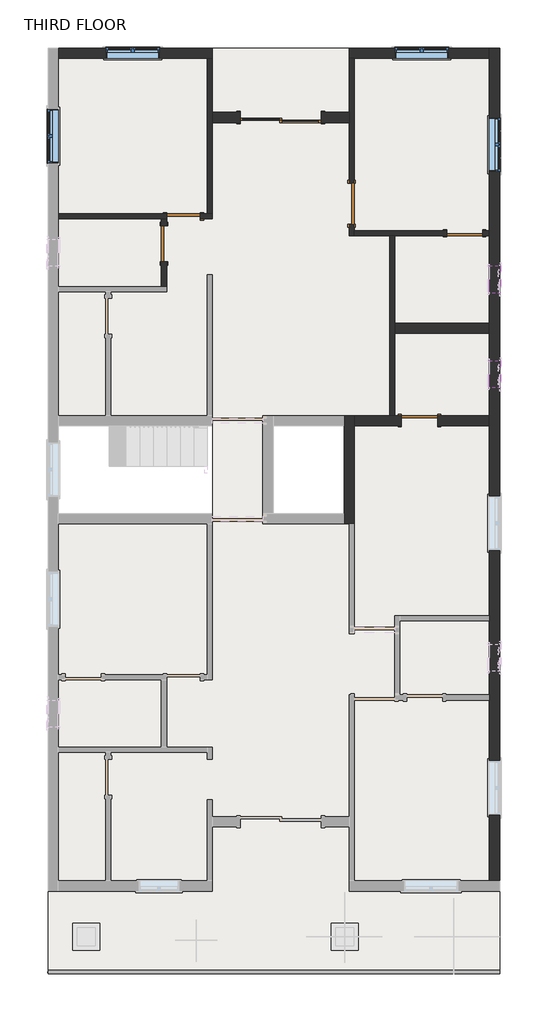
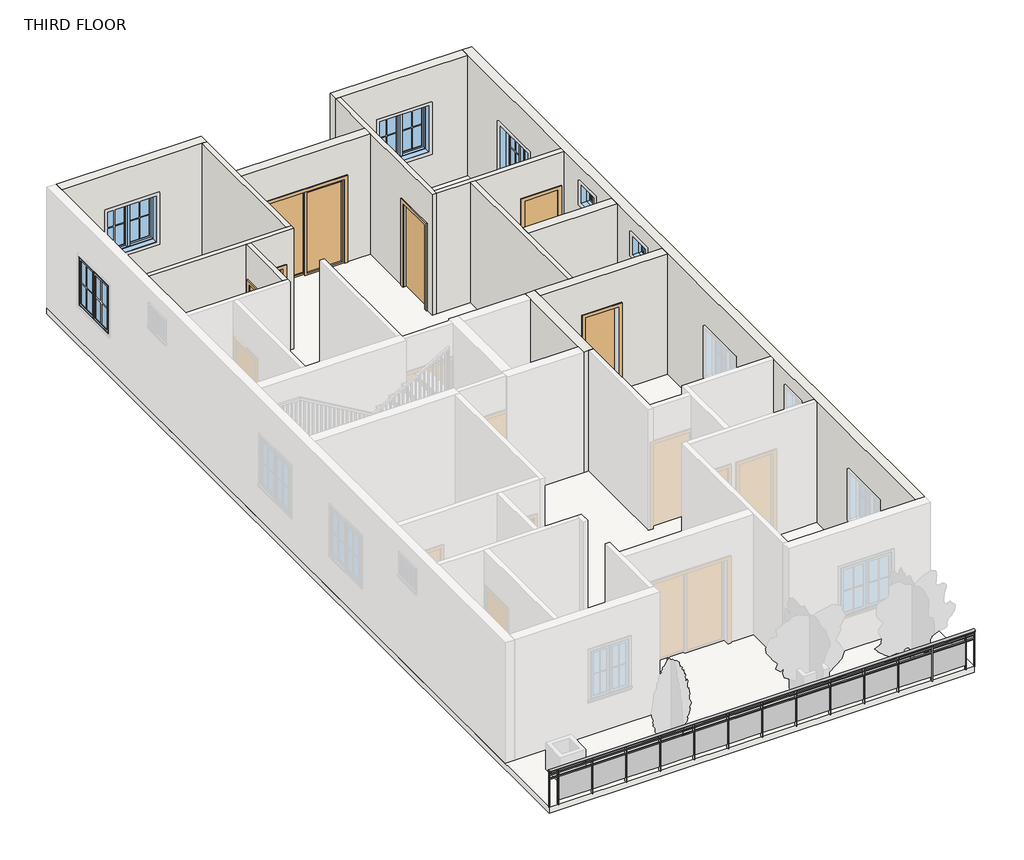
# One storey, part 2 of 4: 13 walls, 6 doors, 6 windows, 1 railing, 1 slab.
"""IFC4 building model written with IfcOpenShell, lengths in millimetres."""

from ifc_helpers import new_model, si_unit, point, frame, origin, place, context, project, spatial, polyline, ellipse_curve, trimmed, outline, extrude, faceted_brep, transform, mapped, element, save
from ifc_brep_helpers import plane_surface, extruded_surface, advanced_brep
from components import door_d4d75d1e, door_214872d5, door_d141acb4, door_38851409, door_7b345704, single_flush_3_x7_e5f9f3c4, window_79894727, window_casement_double_4_x4_af3140d2

model = new_model("IFC4")

# Units and contexts
model_context = context("Model", 3, world=origin())
ifc_project = project(units=[si_unit("LENGTHUNIT", "METRE", prefix="MILLI")], contexts=[model_context])

# Site, building, storey
site = spatial("IfcSite", under=ifc_project)
building = spatial("IfcBuilding", under=site)
storey = spatial("IfcBuildingStorey", under=building, Name="THIRD FLOOR", Elevation=9601.2)

# Doors
placement = place(None, origin())
door_shape = door_d4d75d1e(model_context)
element("IfcDoor", 1, ObjectType="Door-Double-Sliding : 72\" x 84\"", at=placement, inside=storey, context=model_context, shape_type="MappedRepresentation", body=[
    mapped(door_shape, transform((-1119.4789041, 8623.7153263, 9601.2), x_axis=(-1.0, 0.0, 0.0), y_axis=(0.0, -1.0, 0.0), z_axis=(0.0, 0.0, 1.0))),
])
door_2_shape = door_214872d5(model_context)
element("IfcDoor", 2, ObjectType="Single-Flush : 2'6\"X7'", at=placement, inside=storey, context=model_context, shape_type="MappedRepresentation", body=[
    mapped(door_2_shape, transform((-3310.2289041, 6267.8653263, 9601.2), x_axis=(1.0, 0.0, 0.0), y_axis=(0.0, 1.0, 0.0), z_axis=(0.0, 0.0, 1.0))),
])
door_3_shape = door_d141acb4(model_context)
element("IfcDoor", 3, ObjectType="Single-Flush : 2'8\"X7'", at=placement, inside=storey, context=model_context, shape_type="MappedRepresentation", body=[
    mapped(door_3_shape, transform((-3748.3789041, 5651.9153263, 9601.2), x_axis=(0.0, 1.0, 0.0), y_axis=(-1.0, 0.0, 0.0), z_axis=(0.0, 0.0, 1.0))),
])
door_4_shape = door_38851409(model_context)
element("IfcDoor", 4, ObjectType="Single-Flush : 2'8\"X7'", at=placement, inside=storey, context=model_context, shape_type="MappedRepresentation", body=[
    mapped(door_4_shape, transform((3027.0710959, 5886.8653263, 9601.2), x_axis=(1.0, 0.0, 0.0), y_axis=(0.0, 1.0, 0.0), z_axis=(0.0, 0.0, 1.0))),
])
door_5_shape = door_7b345704(model_context)
element("IfcDoor", 5, ObjectType="Single-Flush : 2'8\"X7'", at=placement, inside=storey, context=model_context, shape_type="MappedRepresentation", body=[
    mapped(door_5_shape, transform((2011.0710959, 1664.1153263, 9601.2), x_axis=(-1.0, 0.0, 0.0), y_axis=(0.0, -1.0, 0.0), z_axis=(0.0, 0.0, 1.0))),
])
single_flush_3_x7_shape = single_flush_3_x7_e5f9f3c4(model_context)
element("IfcDoor", 6, ObjectType="Single-Flush : 3'X7'", at=placement, inside=storey, context=model_context, shape_type="MappedRepresentation", body=[
    mapped(single_flush_3_x7_shape, transform((480.7210959, 6553.6153263, 9601.2), x_axis=(0.0, -1.0, 0.0), y_axis=(1.0, 0.0, 0.0), z_axis=(0.0, 0.0, 1.0))),
])

# Railing
element("IfcRailing", 7, ObjectType="Glass Panel - Bottom Fill", at=placement, inside=storey, context=model_context, shape_type="SolidModel", body=[
    advanced_brep(
    [(-6358.2289041, -10731.0846737, 10515.6), (-6358.2289041, -10807.2846737, 10515.6), (3814.4710959, -10731.0846737, 10515.6), (3814.4710959, -10807.2846737, 10515.6)],
    [
        (0, 1, ellipse_curve(frame((-6358.2289041, -10769.1846737, 10515.6), z_axis=(-1.0, 0.0, 0.0), x_axis=(0.0, -1.0, 0.0)), 38.1, 28.575)),
        (1, 0, ellipse_curve(frame((-6358.2289041, -10769.1846737, 10515.6), z_axis=(-1.0, 0.0, 0.0), x_axis=(0.0, -1.0, 0.0)), 38.1, 28.575)),
        (2, 3, ellipse_curve(frame((3814.4710959, -10769.1846737, 10515.6), z_axis=(1.0, 0.0, 0.0), x_axis=(0.0, -1.0, 0.0)), 38.1, 28.575)),
        (3, 2, ellipse_curve(frame((3814.4710959, -10769.1846737, 10515.6), z_axis=(1.0, 0.0, 0.0), x_axis=(0.0, -1.0, 0.0)), 38.1, 28.575)),
        (0, 2),
        (3, 1),
    ],
    [
        plane_surface(frame((-6358.2289041, -10769.1846737, 10515.6), z_axis=(-1.0, 0.0, 0.0), x_axis=(0.0, 1.0, 0.0))),
        plane_surface(frame((3814.4710959, -10769.1846737, 10515.6), z_axis=(1.0, 0.0, 0.0), x_axis=(0.0, 1.0, 0.0))),
        extruded_surface(trimmed(ellipse_curve(frame((3814.4710959, -10769.1846737, 10515.6), z_axis=(-1.0, 0.0, 0.0), x_axis=(0.0, -1.0, 0.0)), 38.1, 28.575), [point((3814.4710959, -10731.0846737, 10515.6))], [point((3814.4710959, -10807.2846737, 10515.6))], True, "CARTESIAN"), (-10172.7, 0.0, 0.0), 10172.7),
        extruded_surface(trimmed(ellipse_curve(frame((3814.4710959, -10769.1846737, 10515.6), z_axis=(-1.0, 0.0, 0.0), x_axis=(0.0, -1.0, 0.0)), 38.1, 28.575), [point((3814.4710959, -10807.2846737, 10515.6))], [point((3814.4710959, -10731.0846737, 10515.6))], True, "CARTESIAN"), (-10172.7, 0.0, 0.0), 10172.7),
    ],
    [
        (0, [[1, 2]]),
        (1, [[3, 4]]),
        (2, [[-1, 5, -4, 6]]),
        (3, [[-2, -6, -3, -5]]),
    ],
),
    extrude(outline(polyline([(-6358.2289041, -10781.8846737), (-6358.2289041, -10756.4846737), (3814.4710959, -10756.4846737), (3814.4710959, -10781.8846737), (-6358.2289041, -10781.8846737)])), frame((0.0, 0.0, 10401.3), z_axis=(0.0, 0.0, 1.0), x_axis=(1.0, 0.0, 0.0)), (0.0, 0.0, 1.0), 25.4),
    extrude(outline(polyline([(-6358.2289041, -10781.8846737), (-6358.2289041, -10756.4846737), (3814.4710959, -10756.4846737), (3814.4710959, -10781.8846737), (-6358.2289041, -10781.8846737)])), frame((0.0, 0.0, 10299.7), z_axis=(0.0, 0.0, 1.0), x_axis=(1.0, 0.0, 0.0)), (0.0, 0.0, 1.0), 25.4),
    extrude(outline(polyline([(3598.5710959, -10794.5846737), (3598.5710959, -10743.7846737), (3611.2710959, -10743.7846737), (3611.2710959, -10794.5846737), (3598.5710959, -10794.5846737)])), frame((0.0, 0.0, 9601.2), z_axis=(0.0, 0.0, 1.0), x_axis=(1.0, 0.0, 0.0)), (0.0, 0.0, 1.0), 885.825),
    extrude(outline(polyline([(2792.1210959, -10762.6495167), (3604.9210959, -10762.6495167), (3604.9210959, -10768.9995167), (2792.1210959, -10768.9995167), (2792.1210959, -10762.6495167)])), frame((0.0, 0.0, 9702.8), z_axis=(0.0, 0.0, 1.0), x_axis=(1.0, 0.0, 0.0)), (0.0, 0.0, 1.0), 596.9),
    extrude(outline(polyline([(2785.7710959, -10794.5846737), (2785.7710959, -10743.7846737), (2798.4710959, -10743.7846737), (2798.4710959, -10794.5846737), (2785.7710959, -10794.5846737)])), frame((0.0, 0.0, 9601.2), z_axis=(0.0, 0.0, 1.0), x_axis=(1.0, 0.0, 0.0)), (0.0, 0.0, 1.0), 885.825),
    extrude(outline(polyline([(1979.3210959, -10762.6495167), (2792.1210959, -10762.6495167), (2792.1210959, -10768.9995167), (1979.3210959, -10768.9995167), (1979.3210959, -10762.6495167)])), frame((0.0, 0.0, 9702.8), z_axis=(0.0, 0.0, 1.0), x_axis=(1.0, 0.0, 0.0)), (0.0, 0.0, 1.0), 596.9),
    extrude(outline(polyline([(1972.9710959, -10794.5846737), (1972.9710959, -10743.7846737), (1985.6710959, -10743.7846737), (1985.6710959, -10794.5846737), (1972.9710959, -10794.5846737)])), frame((0.0, 0.0, 9601.2), z_axis=(0.0, 0.0, 1.0), x_axis=(1.0, 0.0, 0.0)), (0.0, 0.0, 1.0), 885.825),
    extrude(outline(polyline([(1166.5210959, -10762.6495167), (1979.3210959, -10762.6495167), (1979.3210959, -10768.9995167), (1166.5210959, -10768.9995167), (1166.5210959, -10762.6495167)])), frame((0.0, 0.0, 9702.8), z_axis=(0.0, 0.0, 1.0), x_axis=(1.0, 0.0, 0.0)), (0.0, 0.0, 1.0), 596.9),
    extrude(outline(polyline([(1160.1710959, -10794.5846737), (1160.1710959, -10743.7846737), (1172.8710959, -10743.7846737), (1172.8710959, -10794.5846737), (1160.1710959, -10794.5846737)])), frame((0.0, 0.0, 9601.2), z_axis=(0.0, 0.0, 1.0), x_axis=(1.0, 0.0, 0.0)), (0.0, 0.0, 1.0), 885.825),
    extrude(outline(polyline([(353.7210959, -10762.6495167), (1166.5210959, -10762.6495167), (1166.5210959, -10768.9995167), (353.7210959, -10768.9995167), (353.7210959, -10762.6495167)])), frame((0.0, 0.0, 9702.8), z_axis=(0.0, 0.0, 1.0), x_axis=(1.0, 0.0, 0.0)), (0.0, 0.0, 1.0), 596.9),
    extrude(outline(polyline([(347.3710959, -10794.5846737), (347.3710959, -10743.7846737), (360.0710959, -10743.7846737), (360.0710959, -10794.5846737), (347.3710959, -10794.5846737)])), frame((0.0, 0.0, 9601.2), z_axis=(0.0, 0.0, 1.0), x_axis=(1.0, 0.0, 0.0)), (0.0, 0.0, 1.0), 885.825),
    extrude(outline(polyline([(-459.0789041, -10762.6495167), (353.7210959, -10762.6495167), (353.7210959, -10768.9995167), (-459.0789041, -10768.9995167), (-459.0789041, -10762.6495167)])), frame((0.0, 0.0, 9702.8), z_axis=(0.0, 0.0, 1.0), x_axis=(1.0, 0.0, 0.0)), (0.0, 0.0, 1.0), 596.9),
    extrude(outline(polyline([(-465.4289041, -10794.5846737), (-465.4289041, -10743.7846737), (-452.7289041, -10743.7846737), (-452.7289041, -10794.5846737), (-465.4289041, -10794.5846737)])), frame((0.0, 0.0, 9601.2), z_axis=(0.0, 0.0, 1.0), x_axis=(1.0, 0.0, 0.0)), (0.0, 0.0, 1.0), 885.825),
    extrude(outline(polyline([(-1271.8789041, -10762.6495167), (-459.0789041, -10762.6495167), (-459.0789041, -10768.9995167), (-1271.8789041, -10768.9995167), (-1271.8789041, -10762.6495167)])), frame((0.0, 0.0, 9702.8), z_axis=(0.0, 0.0, 1.0), x_axis=(1.0, 0.0, 0.0)), (0.0, 0.0, 1.0), 596.9),
    extrude(outline(polyline([(-1278.2289041, -10794.5846737), (-1278.2289041, -10743.7846737), (-1265.5289041, -10743.7846737), (-1265.5289041, -10794.5846737), (-1278.2289041, -10794.5846737)])), frame((0.0, 0.0, 9601.2), z_axis=(0.0, 0.0, 1.0), x_axis=(1.0, 0.0, 0.0)), (0.0, 0.0, 1.0), 885.825),
    extrude(outline(polyline([(-2084.6789041, -10762.6495167), (-1271.8789041, -10762.6495167), (-1271.8789041, -10768.9995167), (-2084.6789041, -10768.9995167), (-2084.6789041, -10762.6495167)])), frame((0.0, 0.0, 9702.8), z_axis=(0.0, 0.0, 1.0), x_axis=(1.0, 0.0, 0.0)), (0.0, 0.0, 1.0), 596.9),
    extrude(outline(polyline([(-2091.0289041, -10794.5846737), (-2091.0289041, -10743.7846737), (-2078.3289041, -10743.7846737), (-2078.3289041, -10794.5846737), (-2091.0289041, -10794.5846737)])), frame((0.0, 0.0, 9601.2), z_axis=(0.0, 0.0, 1.0), x_axis=(1.0, 0.0, 0.0)), (0.0, 0.0, 1.0), 885.825),
    extrude(outline(polyline([(-2897.4789041, -10762.6495167), (-2084.6789041, -10762.6495167), (-2084.6789041, -10768.9995167), (-2897.4789041, -10768.9995167), (-2897.4789041, -10762.6495167)])), frame((0.0, 0.0, 9702.8), z_axis=(0.0, 0.0, 1.0), x_axis=(1.0, 0.0, 0.0)), (0.0, 0.0, 1.0), 596.9),
    extrude(outline(polyline([(-2903.8289041, -10794.5846737), (-2903.8289041, -10743.7846737), (-2891.1289041, -10743.7846737), (-2891.1289041, -10794.5846737), (-2903.8289041, -10794.5846737)])), frame((0.0, 0.0, 9601.2), z_axis=(0.0, 0.0, 1.0), x_axis=(1.0, 0.0, 0.0)), (0.0, 0.0, 1.0), 885.825),
    extrude(outline(polyline([(-3710.2789041, -10762.6495167), (-2897.4789041, -10762.6495167), (-2897.4789041, -10768.9995167), (-3710.2789041, -10768.9995167), (-3710.2789041, -10762.6495167)])), frame((0.0, 0.0, 9702.8), z_axis=(0.0, 0.0, 1.0), x_axis=(1.0, 0.0, 0.0)), (0.0, 0.0, 1.0), 596.9),
    extrude(outline(polyline([(-3716.6289041, -10794.5846737), (-3716.6289041, -10743.7846737), (-3703.9289041, -10743.7846737), (-3703.9289041, -10794.5846737), (-3716.6289041, -10794.5846737)])), frame((0.0, 0.0, 9601.2), z_axis=(0.0, 0.0, 1.0), x_axis=(1.0, 0.0, 0.0)), (0.0, 0.0, 1.0), 885.825),
    extrude(outline(polyline([(-4523.0789041, -10762.6495167), (-3710.2789041, -10762.6495167), (-3710.2789041, -10768.9995167), (-4523.0789041, -10768.9995167), (-4523.0789041, -10762.6495167)])), frame((0.0, 0.0, 9702.8), z_axis=(0.0, 0.0, 1.0), x_axis=(1.0, 0.0, 0.0)), (0.0, 0.0, 1.0), 596.9),
    extrude(outline(polyline([(-4529.4289041, -10794.5846737), (-4529.4289041, -10743.7846737), (-4516.7289041, -10743.7846737), (-4516.7289041, -10794.5846737), (-4529.4289041, -10794.5846737)])), frame((0.0, 0.0, 9601.2), z_axis=(0.0, 0.0, 1.0), x_axis=(1.0, 0.0, 0.0)), (0.0, 0.0, 1.0), 885.825),
    extrude(outline(polyline([(-5335.8789041, -10762.6495167), (-4523.0789041, -10762.6495167), (-4523.0789041, -10768.9995167), (-5335.8789041, -10768.9995167), (-5335.8789041, -10762.6495167)])), frame((0.0, 0.0, 9702.8), z_axis=(0.0, 0.0, 1.0), x_axis=(1.0, 0.0, 0.0)), (0.0, 0.0, 1.0), 596.9),
    extrude(outline(polyline([(-5342.2289041, -10794.5846737), (-5342.2289041, -10743.7846737), (-5329.5289041, -10743.7846737), (-5329.5289041, -10794.5846737), (-5342.2289041, -10794.5846737)])), frame((0.0, 0.0, 9601.2), z_axis=(0.0, 0.0, 1.0), x_axis=(1.0, 0.0, 0.0)), (0.0, 0.0, 1.0), 885.825),
    extrude(outline(polyline([(-6148.6789041, -10762.6495167), (-5335.8789041, -10762.6495167), (-5335.8789041, -10768.9995167), (-6148.6789041, -10768.9995167), (-6148.6789041, -10762.6495167)])), frame((0.0, 0.0, 9702.8), z_axis=(0.0, 0.0, 1.0), x_axis=(1.0, 0.0, 0.0)), (0.0, 0.0, 1.0), 596.9),
    extrude(outline(polyline([(-6155.0289041, -10794.5846737), (-6155.0289041, -10743.7846737), (-6142.3289041, -10743.7846737), (-6142.3289041, -10794.5846737), (-6155.0289041, -10794.5846737)])), frame((0.0, 0.0, 9601.2), z_axis=(0.0, 0.0, 1.0), x_axis=(1.0, 0.0, 0.0)), (0.0, 0.0, 1.0), 885.825),
    extrude(outline(polyline([(3801.7710959, -10778.7096737), (3801.7710959, -10759.6596737), (3820.8210959, -10759.6596737), (3820.8210959, -10778.7096737), (3801.7710959, -10778.7096737)])), frame((0.0, 0.0, 9601.2), z_axis=(0.0, 0.0, 1.0), x_axis=(1.0, 0.0, 0.0)), (0.0, 0.0, 1.0), 885.825),
    extrude(outline(polyline([(-6364.5789041, -10778.7096737), (-6364.5789041, -10759.6596737), (-6345.5289041, -10759.6596737), (-6345.5289041, -10778.7096737), (-6364.5789041, -10778.7096737)])), frame((0.0, 0.0, 9601.2), z_axis=(0.0, 0.0, 1.0), x_axis=(1.0, 0.0, 0.0)), (0.0, 0.0, 1.0), 885.825),
])

# Slab
element("IfcSlab", 8, ObjectType="6\"", at=placement, inside=storey, context=model_context, shape_type="SweptSolid", body=[
    extrude(outline(polyline([(3814.4710959, 10058.8153263), (3814.4710959, -10769.1846737), (-6358.2289041, -10769.1846737), (-6358.2289041, 10058.8153263), (3814.4710959, 10058.8153263)]), holes=[polyline([(-2662.5289041, 1549.8153263), (-6129.6289041, 1549.8153263), (-6129.6289041, -431.3846737), (-2662.5289041, -431.3846737), (-2662.5289041, 1549.8153263)]), polyline([(537.8710959, 1778.4153263), (-1519.5289041, 1778.4153263), (-1519.5289041, -659.9846737), (537.8710959, -659.9846737), (537.8710959, 1778.4153263)])]), frame((0.0, 0.0, 9448.8), z_axis=(0.0, 0.0, 1.0), x_axis=(1.0, 0.0, 0.0)), (0.0, 0.0, 1.0), 152.4),
])

# Walls
element("IfcWall", 9, ObjectType="4.5\"", at=placement, inside=storey, context=model_context, shape_type="SweptSolid", body=[
    extrude(outline(polyline([(6210.7153263, 9601.2), (6058.3153263, 9601.2), (6058.3153263, 11734.8), (5245.5153263, 11734.8), (5245.5153263, 9601.2), (4686.7153263, 9601.2), (4686.7153263, 12649.2), (6210.7153263, 12649.2), (6210.7153263, 9601.2)])), frame((-3805.5289041, 0.0, 0.0), z_axis=(1.0, 0.0, 0.0), x_axis=(0.0, 1.0, 0.0)), (0.0, 0.0, 1.0), 114.3),
])
element("IfcWall", 10, ObjectType="4.5\"", at=placement, inside=storey, context=model_context, shape_type="Brep", body=[
    faceted_brep([(-2929.2289041, 6210.7153263, 11734.8), (-2929.2289041, 6210.7153263, 9601.2), (-2662.5289041, 6210.7153263, 9601.2), (-2662.5289041, 6210.7153263, 12649.2), (-3691.2289041, 6210.7153263, 12649.2), (-3805.5289041, 6210.7153263, 12649.2), (-6129.6289041, 6210.7153263, 12649.2), (-6129.6289041, 6210.7153263, 9601.2), (-3805.5289041, 6210.7153263, 9601.2), (-3691.2289041, 6210.7153263, 9601.2), (-3691.2289041, 6210.7153263, 11734.8), (-2662.5289041, 6325.0153263, 9601.2), (-2776.8289041, 6325.0153263, 9601.2), (-2929.2289041, 6325.0153263, 9601.2), (-2929.2289041, 6325.0153263, 11734.8), (-3691.2289041, 6325.0153263, 11734.8), (-3691.2289041, 6325.0153263, 9601.2), (-6129.6289041, 6325.0153263, 9601.2), (-6129.6289041, 6325.0153263, 12649.2), (-2776.8289041, 6325.0153263, 12649.2), (-2662.5289041, 6325.0153263, 12649.2)], [[[0, 1, 2, 3, 4, 5, 6, 7, 8, 9, 10]], [[11, 12, 13, 14, 15, 16, 17, 18, 19, 20]], [[2, 1, 13, 12, 11]], [[9, 8, 7, 17, 16]], [[6, 5, 4, 3, 20, 19, 18]], [[7, 6, 18, 17]], [[3, 2, 11, 20]], [[14, 13, 1, 0]], [[15, 14, 0, 10]], [[16, 15, 10, 9]]]),
])
element("IfcWall", 11, ObjectType="4.5\"", at=placement, inside=storey, context=model_context, shape_type="Brep", body=[
    faceted_brep([(-2662.5289041, 6325.0153263, 9601.2), (-2662.5289041, 8382.4153263, 9601.2), (-2662.5289041, 8611.0153263, 9601.2), (-2662.5289041, 9830.2153263, 9601.2), (-2662.5289041, 9830.2153263, 12649.2), (-2662.5289041, 8611.0153263, 12649.2), (-2662.5289041, 8382.4153263, 12649.2), (-2662.5289041, 6325.0153263, 12649.2), (-2776.8289041, 6325.0153263, 9601.2), (-2776.8289041, 6325.0153263, 12649.2), (-2776.8289041, 9830.2153263, 12649.2), (-2776.8289041, 9830.2153263, 9601.2)], [[[0, 1, 2, 3, 4, 5, 6, 7]], [[8, 9, 10, 11]], [[3, 2, 1, 0, 8, 11]], [[7, 6, 5, 4, 10, 9]], [[0, 7, 9, 8]], [[4, 3, 11, 10]]]),
])
element("IfcWall", 12, ObjectType="4.5\"", at=placement, inside=storey, context=model_context, shape_type="Brep", body=[
    faceted_brep([(423.5710959, 6096.4153263, 11734.8), (423.5710959, 6096.4153263, 9601.2), (423.5710959, 5829.7153263, 9601.2), (423.5710959, 5829.7153263, 12649.2), (423.5710959, 8382.4153263, 12649.2), (423.5710959, 8611.0153263, 12649.2), (423.5710959, 9830.2153263, 12649.2), (423.5710959, 9830.2153263, 9601.2), (423.5710959, 8611.0153263, 9601.2), (423.5710959, 8382.4153263, 9601.2), (423.5710959, 7010.8153263, 9601.2), (423.5710959, 7010.8153263, 11734.8), (537.8710959, 5829.7153263, 9601.2), (537.8710959, 5944.0153263, 9601.2), (537.8710959, 6096.4153263, 9601.2), (537.8710959, 6096.4153263, 11734.8), (537.8710959, 7010.8153263, 11734.8), (537.8710959, 7010.8153263, 9601.2), (537.8710959, 9830.2153263, 9601.2), (537.8710959, 9830.2153263, 12649.2), (537.8710959, 5944.0153263, 12649.2), (537.8710959, 5829.7153263, 12649.2)], [[[0, 1, 2, 3, 4, 5, 6, 7, 8, 9, 10, 11]], [[12, 13, 14, 15, 16, 17, 18, 19, 20, 21]], [[2, 1, 14, 13, 12]], [[10, 9, 8, 7, 18, 17]], [[6, 5, 4, 3, 21, 20, 19]], [[7, 6, 19, 18]], [[3, 2, 12, 21]], [[15, 14, 1, 0]], [[16, 15, 0, 11]], [[17, 16, 11, 10]]]),
])
element("IfcWall", 13, ObjectType="4.5\"", at=placement, inside=storey, context=model_context, shape_type="Brep", body=[
    faceted_brep([(3433.4710959, 5829.7153263, 11734.8), (3433.4710959, 5829.7153263, 9601.2), (3585.8710959, 5829.7153263, 9601.2), (3585.8710959, 5829.7153263, 12649.2), (1452.2710959, 5829.7153263, 12649.2), (1337.9710959, 5829.7153263, 12649.2), (537.8710959, 5829.7153263, 12649.2), (537.8710959, 5829.7153263, 9601.2), (1337.9710959, 5829.7153263, 9601.2), (1452.2710959, 5829.7153263, 9601.2), (2620.6710959, 5829.7153263, 9601.2), (2620.6710959, 5829.7153263, 11734.8), (3585.8710959, 5944.0153263, 9601.2), (3433.4710959, 5944.0153263, 9601.2), (3433.4710959, 5944.0153263, 11734.8), (2620.6710959, 5944.0153263, 11734.8), (2620.6710959, 5944.0153263, 9601.2), (537.8710959, 5944.0153263, 9601.2), (537.8710959, 5944.0153263, 12649.2), (3585.8710959, 5944.0153263, 12649.2)], [[[0, 1, 2, 3, 4, 5, 6, 7, 8, 9, 10, 11]], [[12, 13, 14, 15, 16, 17, 18, 19]], [[2, 1, 13, 12]], [[10, 9, 8, 7, 17, 16]], [[6, 5, 4, 3, 19, 18]], [[7, 6, 18, 17]], [[3, 2, 12, 19]], [[14, 13, 1, 0]], [[15, 14, 0, 11]], [[16, 15, 11, 10]]]),
])
element("IfcWall", 14, ObjectType="4.5\"", at=placement, inside=storey, context=model_context, shape_type="Brep", body=[
    faceted_brep([(1337.9710959, 5829.7153263, 9601.2), (1337.9710959, 1778.4153263, 9601.2), (1337.9710959, 1778.4153263, 12649.2), (1337.9710959, 5829.7153263, 12649.2), (1452.2710959, 5829.7153263, 9601.2), (1452.2710959, 5829.7153263, 12649.2), (1452.2710959, 3861.2153263, 12649.2), (1452.2710959, 3632.6153263, 12649.2), (1452.2710959, 1778.4153263, 12649.2), (1452.2710959, 1778.4153263, 9601.2), (1452.2710959, 3632.6153263, 9601.2), (1452.2710959, 3861.2153263, 9601.2)], [[[0, 1, 2, 3]], [[4, 5, 6, 7, 8, 9, 10, 11]], [[1, 0, 4, 11, 10, 9]], [[3, 2, 8, 7, 6, 5]], [[2, 1, 9, 8]], [[0, 3, 5, 4]]]),
])
element("IfcWall", 15, ObjectType="9\"", at=placement, inside=storey, context=model_context, shape_type="Brep", body=[
    faceted_brep([(3814.4710959, -8711.7846737, 9601.2), (3814.4710959, 10058.8153263, 9601.2), (3814.4710959, 10058.8153263, 12649.2), (3814.4710959, -8711.7846737, 12649.2), (3814.4710959, -7225.8846737, 11734.8), (3814.4710959, -6006.6846737, 11734.8), (3814.4710959, -6006.6846737, 10515.6), (3814.4710959, -7225.8846737, 10515.6), (3814.4710959, -1256.8846737, 11734.8), (3814.4710959, -37.6846737, 11734.8), (3814.4710959, -37.6846737, 10515.6), (3814.4710959, -1256.8846737, 10515.6), (3814.4710959, 7277.5153263, 11734.8), (3814.4710959, 8496.7153263, 11734.8), (3814.4710959, 8496.7153263, 10515.6), (3814.4710959, 7277.5153263, 10515.6), (3814.4710959, -3987.3846737, 12268.2), (3814.4710959, -3377.7846737, 12268.2), (3814.4710959, -3377.7846737, 11734.8), (3814.4710959, -3987.3846737, 11734.8), (3814.4710959, 2400.7153263, 12268.2), (3814.4710959, 3010.3153263, 12268.2), (3814.4710959, 3010.3153263, 11734.8), (3814.4710959, 2400.7153263, 11734.8), (3814.4710959, 4540.6653263, 12268.2), (3814.4710959, 5150.2653263, 12268.2), (3814.4710959, 5150.2653263, 11734.8), (3814.4710959, 4540.6653263, 11734.8), (3585.8710959, -8711.7846737, 9601.2), (3585.8710959, -8711.7846737, 12649.2), (3585.8710959, -4635.0846737, 12649.2), (3585.8710959, -4520.7846737, 12649.2), (3585.8710959, -2844.3846737, 12649.2), (3585.8710959, -2730.0846737, 12649.2), (3585.8710959, 1549.8153263, 12649.2), (3585.8710959, 1778.4153263, 12649.2), (3585.8710959, 3632.6153263, 12649.2), (3585.8710959, 3861.2153263, 12649.2), (3585.8710959, 5829.7153263, 12649.2), (3585.8710959, 5944.0153263, 12649.2), (3585.8710959, 9830.2153263, 12649.2), (3585.8710959, 10058.8153263, 12649.2), (3585.8710959, 10058.8153263, 9601.2), (3585.8710959, 9830.2153263, 9601.2), (3585.8710959, 5944.0153263, 9601.2), (3585.8710959, 5829.7153263, 9601.2), (3585.8710959, 3861.2153263, 9601.2), (3585.8710959, 3632.6153263, 9601.2), (3585.8710959, 1778.4153263, 9601.2), (3585.8710959, 1549.8153263, 9601.2), (3585.8710959, -2730.0846737, 9601.2), (3585.8710959, -2844.3846737, 9601.2), (3585.8710959, -4520.7846737, 9601.2), (3585.8710959, -4635.0846737, 9601.2), (3585.8710959, -7225.8846737, 11734.8), (3585.8710959, -7225.8846737, 10515.6), (3585.8710959, -6006.6846737, 10515.6), (3585.8710959, -6006.6846737, 11734.8), (3585.8710959, -1256.8846737, 11734.8), (3585.8710959, -1256.8846737, 10515.6), (3585.8710959, -37.6846737, 10515.6), (3585.8710959, -37.6846737, 11734.8), (3585.8710959, 7277.5153263, 11734.8), (3585.8710959, 7277.5153263, 10515.6), (3585.8710959, 8496.7153263, 10515.6), (3585.8710959, 8496.7153263, 11734.8), (3585.8710959, -3987.3846737, 12268.2), (3585.8710959, -3987.3846737, 11734.8), (3585.8710959, -3377.7846737, 11734.8), (3585.8710959, -3377.7846737, 12268.2), (3585.8710959, 2400.7153263, 12268.2), (3585.8710959, 2400.7153263, 11734.8), (3585.8710959, 3010.3153263, 11734.8), (3585.8710959, 3010.3153263, 12268.2), (3585.8710959, 4540.6653263, 12268.2), (3585.8710959, 4540.6653263, 11734.8), (3585.8710959, 5150.2653263, 11734.8), (3585.8710959, 5150.2653263, 12268.2)], [[[0, 1, 2, 3], [4, 5, 6, 7], [8, 9, 10, 11], [12, 13, 14, 15], [16, 17, 18, 19], [20, 21, 22, 23], [24, 25, 26, 27]], [[28, 29, 30, 31, 32, 33, 34, 35, 36, 37, 38, 39, 40, 41, 42, 43, 44, 45, 46, 47, 48, 49, 50, 51, 52, 53], [54, 55, 56, 57], [58, 59, 60, 61], [62, 63, 64, 65], [66, 67, 68, 69], [70, 71, 72, 73], [74, 75, 76, 77]], [[1, 0, 28, 53, 52, 51, 50, 49, 48, 47, 46, 45, 44, 43, 42]], [[3, 2, 41, 40, 39, 38, 37, 36, 35, 34, 33, 32, 31, 30, 29]], [[0, 3, 29, 28]], [[2, 1, 42, 41]], [[55, 54, 4, 7]], [[56, 55, 7, 6]], [[57, 56, 6, 5]], [[54, 57, 5, 4]], [[59, 58, 8, 11]], [[60, 59, 11, 10]], [[61, 60, 10, 9]], [[58, 61, 9, 8]], [[63, 62, 12, 15]], [[64, 63, 15, 14]], [[65, 64, 14, 13]], [[62, 65, 13, 12]], [[67, 66, 16, 19]], [[68, 67, 19, 18]], [[69, 68, 18, 17]], [[66, 69, 17, 16]], [[71, 70, 20, 23]], [[72, 71, 23, 22]], [[73, 72, 22, 21]], [[70, 73, 21, 20]], [[75, 74, 24, 27]], [[76, 75, 27, 26]], [[77, 76, 26, 25]], [[74, 77, 25, 24]]]),
])
element("IfcWall", 16, ObjectType="9\"", at=placement, inside=storey, context=model_context, shape_type="Brep", body=[
    faceted_brep([(3585.8710959, 10058.8153263, 9601.2), (423.5710959, 10058.8153263, 9601.2), (423.5710959, 10058.8153263, 12649.2), (3585.8710959, 10058.8153263, 12649.2), (2671.4710959, 10058.8153263, 11734.8), (1452.2710959, 10058.8153263, 11734.8), (1452.2710959, 10058.8153263, 10515.6), (2671.4710959, 10058.8153263, 10515.6), (3585.8710959, 9830.2153263, 9601.2), (3585.8710959, 9830.2153263, 12649.2), (537.8710959, 9830.2153263, 12649.2), (423.5710959, 9830.2153263, 12649.2), (423.5710959, 9830.2153263, 9601.2), (537.8710959, 9830.2153263, 9601.2), (2671.4710959, 9830.2153263, 11734.8), (2671.4710959, 9830.2153263, 10515.6), (1452.2710959, 9830.2153263, 10515.6), (1452.2710959, 9830.2153263, 11734.8)], [[[0, 1, 2, 3], [4, 5, 6, 7]], [[8, 9, 10, 11, 12, 13], [14, 15, 16, 17]], [[1, 0, 8, 13, 12]], [[3, 2, 11, 10, 9]], [[0, 3, 9, 8]], [[2, 1, 12, 11]], [[15, 14, 4, 7]], [[16, 15, 7, 6]], [[17, 16, 6, 5]], [[14, 17, 5, 4]]]),
])
element("IfcWall", 17, ObjectType="9\"", at=placement, inside=storey, context=model_context, shape_type="Brep", body=[
    faceted_brep([(-2662.5289041, 10058.8153263, 9601.2), (-6129.6289041, 10058.8153263, 9601.2), (-6129.6289041, 10058.8153263, 12649.2), (-2662.5289041, 10058.8153263, 12649.2), (-3843.6289041, 10058.8153263, 11734.8), (-5062.8289041, 10058.8153263, 11734.8), (-5062.8289041, 10058.8153263, 10515.6), (-3843.6289041, 10058.8153263, 10515.6), (-2662.5289041, 9830.2153263, 9601.2), (-2662.5289041, 9830.2153263, 12649.2), (-2776.8289041, 9830.2153263, 12649.2), (-6129.6289041, 9830.2153263, 12649.2), (-6129.6289041, 9830.2153263, 9601.2), (-2776.8289041, 9830.2153263, 9601.2), (-3843.6289041, 9830.2153263, 11734.8), (-3843.6289041, 9830.2153263, 10515.6), (-5062.8289041, 9830.2153263, 10515.6), (-5062.8289041, 9830.2153263, 11734.8)], [[[0, 1, 2, 3], [4, 5, 6, 7]], [[8, 9, 10, 11, 12, 13], [14, 15, 16, 17]], [[1, 0, 8, 13, 12]], [[3, 2, 11, 10, 9]], [[2, 1, 12, 11]], [[0, 3, 9, 8]], [[15, 14, 4, 7]], [[16, 15, 7, 6]], [[17, 16, 6, 5]], [[14, 17, 5, 4]]]),
])
element("IfcWall", 18, ObjectType="9\"", at=placement, inside=storey, context=model_context, shape_type="Brep", body=[
    faceted_brep([(309.2710959, 1778.4153263, 9601.2), (309.2710959, 1549.8153263, 9601.2), (309.2710959, -431.3846737, 9601.2), (309.2710959, -659.9846737, 9601.2), (309.2710959, -659.9846737, 12649.2), (309.2710959, -431.3846737, 12649.2), (309.2710959, 1549.8153263, 12649.2), (309.2710959, 1778.4153263, 12649.2), (537.8710959, 1778.4153263, 9601.2), (537.8710959, 1778.4153263, 12649.2), (537.8710959, 1549.8153263, 12649.2), (537.8710959, -659.9846737, 12649.2), (537.8710959, -659.9846737, 9601.2), (537.8710959, 1549.8153263, 9601.2), (423.5710959, -659.9846737, 9601.2), (423.5710959, -659.9846737, 12649.2)], [[[0, 1, 2, 3, 4, 5, 6, 7]], [[8, 9, 10, 11, 12, 13]], [[3, 2, 1, 0, 8, 13, 12, 14]], [[7, 6, 5, 4, 15, 11, 10, 9]], [[4, 3, 14, 12, 11, 15]], [[0, 7, 9, 8]]]),
])
element("IfcWall", 19, ObjectType="9\"", at=placement, inside=storey, context=model_context, shape_type="Brep", body=[
    faceted_brep([(537.8710959, 1549.8153263, 9601.2), (1604.6710959, 1549.8153263, 9601.2), (1604.6710959, 1549.8153263, 11734.8), (2417.4710959, 1549.8153263, 11734.8), (2417.4710959, 1549.8153263, 9601.2), (3585.8710959, 1549.8153263, 9601.2), (3585.8710959, 1549.8153263, 12649.2), (537.8710959, 1549.8153263, 12649.2), (1604.6710959, 1778.4153263, 11734.8), (1604.6710959, 1778.4153263, 9601.2), (1452.2710959, 1778.4153263, 9601.2), (1337.9710959, 1778.4153263, 9601.2), (537.8710959, 1778.4153263, 9601.2), (537.8710959, 1778.4153263, 12649.2), (1337.9710959, 1778.4153263, 12649.2), (1452.2710959, 1778.4153263, 12649.2), (3585.8710959, 1778.4153263, 12649.2), (3585.8710959, 1778.4153263, 9601.2), (2417.4710959, 1778.4153263, 9601.2), (2417.4710959, 1778.4153263, 11734.8)], [[[0, 1, 2, 3, 4, 5, 6, 7]], [[8, 9, 10, 11, 12, 13, 14, 15, 16, 17, 18, 19]], [[18, 17, 5, 4]], [[12, 11, 10, 9, 1, 0]], [[7, 6, 16, 15, 14, 13]], [[0, 7, 13, 12]], [[6, 5, 17, 16]], [[2, 1, 9, 8]], [[3, 2, 8, 19]], [[4, 3, 19, 18]]]),
])
element("IfcWall", 20, ObjectType="9\"", at=placement, inside=storey, context=model_context, shape_type="SweptSolid", body=[
    extrude(outline(polyline([(1452.2710959, 3861.2153263), (3585.8710959, 3861.2153263), (3585.8710959, 3632.6153263), (1452.2710959, 3632.6153263), (1452.2710959, 3861.2153263)])), frame((0.0, 0.0, 9601.2), z_axis=(0.0, 0.0, 1.0), x_axis=(1.0, 0.0, 0.0)), (0.0, 0.0, 1.0), 3048.0),
])
element("IfcWall", 21, ObjectType="9\"", at=placement, inside=storey, context=model_context, shape_type="SweptSolid", body=[
    extrude(outline(polyline([(9601.2, -2662.5289041), (9601.2, -2033.8789041), (11734.8, -2033.8789041), (11734.8, -205.0789041), (9601.2, -205.0789041), (9601.2, 423.5710959), (12649.2, 423.5710959), (12649.2, -2662.5289041), (9601.2, -2662.5289041)])), frame((0.0, 8382.4153263, 0.0), z_axis=(0.0, 1.0, 0.0), x_axis=(0.0, 0.0, 1.0)), (0.0, 0.0, 1.0), 228.6),
])

# Windows
window_shape = window_79894727(model_context)
element("IfcWindow", 22, ObjectType="Window-Casement-Double : 2'X1'9\"", at=placement, inside=storey, context=model_context, shape_type="MappedRepresentation", body=[
    mapped(window_shape, transform((3700.1710959, 2705.5153263, 9601.2), x_axis=(0.0, -1.0, 0.0), y_axis=(1.0, 0.0, 0.0), z_axis=(0.0, 0.0, 1.0))),
])
element("IfcWindow", 23, ObjectType="Window-Casement-Double : 2'X1'9\"", at=placement, inside=storey, context=model_context, shape_type="MappedRepresentation", body=[
    mapped(window_shape, transform((3700.1710959, 4845.4653263, 9601.2), x_axis=(0.0, -1.0, 0.0), y_axis=(1.0, 0.0, 0.0), z_axis=(0.0, 0.0, 1.0))),
])
window_casement_double_4_x4_shape = window_casement_double_4_x4_af3140d2(model_context)
element("IfcWindow", 24, ObjectType="Window-Casement-Double : 4'X4'", at=placement, inside=storey, context=model_context, shape_type="MappedRepresentation", body=[
    mapped(window_casement_double_4_x4_shape, transform((-4453.2289041, 9944.5153263, 9601.2), x_axis=(1.0, 0.0, 0.0), y_axis=(0.0, 1.0, 0.0), z_axis=(0.0, 0.0, 1.0))),
])
element("IfcWindow", 25, ObjectType="Window-Casement-Double : 4'X4'", at=placement, inside=storey, context=model_context, shape_type="MappedRepresentation", body=[
    mapped(window_casement_double_4_x4_shape, transform((-6243.9289041, 8077.6153263, 9601.2), x_axis=(0.0, 1.0, 0.0), y_axis=(-1.0, 0.0, 0.0), z_axis=(0.0, 0.0, 1.0))),
])
element("IfcWindow", 26, ObjectType="Window-Casement-Double : 4'X4'", at=placement, inside=storey, context=model_context, shape_type="MappedRepresentation", body=[
    mapped(window_casement_double_4_x4_shape, transform((3700.1710959, 7887.1153263, 9601.2), x_axis=(0.0, -1.0, 0.0), y_axis=(1.0, 0.0, 0.0), z_axis=(0.0, 0.0, 1.0))),
])
element("IfcWindow", 27, ObjectType="Window-Casement-Double : 4'X4'", at=placement, inside=storey, context=model_context, shape_type="MappedRepresentation", body=[
    mapped(window_casement_double_4_x4_shape, transform((2061.8710959, 9944.5153263, 9601.2), x_axis=(1.0, 0.0, 0.0), y_axis=(0.0, 1.0, 0.0), z_axis=(0.0, 0.0, 1.0))),
])

save(model, "model.ifc")

# Revit data of these elements
# Type "Door-Double-Sliding : 72\" x 84\""
#   Type Mark = "14"
#   Construction Type Id = "opn-d45"
#   Assembly Code = "C1020"
#   Analytic Construction = "Wood frame, double glass door "
#   Thickness = 0' - 2"
#   Thermal Resistance (R) = 1.8150 (h·ft²·°F)/BTU
#   Heat Transfer Coefficient (U) = 0.5510 BTU/(h·ft²·°F)
#   Height = 7' - 0"
#   Rail Width = 0' - 2"
#   Stiles = 0' - 2"
#   Trim Projection Ext = 0' - 1"
#   Trim Projection Int = 0' - 1"
#   Trim Width = 0' - 3"
#   Width = 6' - 0"
#   Define Thermal Properties by = 1
#   Glazing = Glass
#   Panel Material = Wood - Birch - Solid Stained Light Low Gloss
#   Trim Material = Paint - Sienna
#   Visual Light Transmittance = 0
#   Solar Heat Gain Coefficient = 0
#   Function = (empty or 0)
#   Wall Closure = (empty or 0)
# Type "Single-Flush : 2'6\"X7'"
#   Type Mark = "13"
#   Construction Type Id = "MDOOR"
#   Assembly Code = "C1020"
#   Analytic Construction = "Metal"
#   Thickness = 0' - 2"
#   Heat Transfer Coefficient (U) = 0.651978 BTU/(h·ft²·°F)
#   Height = 7' - 0"
#   Trim Projection Ext = 0' - 1"
#   Trim Projection Int = 0' - 1"
#   Trim Width = 0' - 3"
#   Width = 2' - 6"
#   Define Thermal Properties by = 1
#   Door Material = Door - Panel
#   Frame Material = Door - Frame
#   Visual Light Transmittance = 0
#   Solar Heat Gain Coefficient = 0
#   Function = (empty or 0)
#   Wall Closure = (empty or 0)
# Type "Single-Flush : 2'8\"X7'"
#   Type Mark = "12"
#   Construction Type Id = "MDOOR"
#   Assembly Code = "C1020"
#   Analytic Construction = "Metal"
#   Thickness = 0' - 2"
#   Heat Transfer Coefficient (U) = 0.651978 BTU/(h·ft²·°F)
#   Height = 7' - 0"
#   Trim Projection Ext = 0' - 1"
#   Trim Projection Int = 0' - 1"
#   Trim Width = 0' - 3"
#   Width = 2' - 8"
#   Define Thermal Properties by = 1
#   Door Material = Door - Panel
#   Frame Material = Door - Frame
#   Visual Light Transmittance = 0
#   Solar Heat Gain Coefficient = 0
#   Function = (empty or 0)
#   Wall Closure = (empty or 0)
# Type "Single-Flush : 3'X7'"
#   Type Mark = "8"
#   Construction Type Id = "MDOOR"
#   Assembly Code = "C1020"
#   Analytic Construction = "Metal"
#   Thickness = 0' - 2"
#   Heat Transfer Coefficient (U) = 0.651978 BTU/(h·ft²·°F)
#   Height = 7' - 0"
#   Trim Projection Ext = 0' - 1"
#   Trim Projection Int = 0' - 1"
#   Trim Width = 0' - 3"
#   Width = 3' - 0"
#   Define Thermal Properties by = 1
#   Door Material = Door - Panel
#   Frame Material = Door - Frame
#   Visual Light Transmittance = 0
#   Solar Heat Gain Coefficient = 0
#   Function = (empty or 0)
#   Wall Closure = (empty or 0)
# Type "Glass Panel - Bottom Fill"
#   Assembly Code = "C2010400"
#   built-in parameter 1008612 = 0.0416667 (stored number, unit not read)
#   built-in parameter 1008611 = 0.0416667 (stored number, unit not read)
#   built-in parameter 1008609 = 0.333333 (stored number, unit not read)
#   built-in parameter 1008604 = 0.166667 (stored number, unit not read)
#   built-in parameter 1008603 = 0.166667 (stored number, unit not read)
#   Railing Height = 3' - 0"
#   built-in parameter 1008630 = 2
#   built-in parameter 1008610 = 2
#   built-in parameter 1008618 = Baluster - Square : 3/4"
# Type "6\""
#   Assembly Code = "B1010"
#   Function = 0
#   Layers, outside or top first: 0' - 6" no material (function 1)
# Type "4.5\""
#   Assembly Code = "B2010"
#   Layers, outside or top first: 0' - 4 1/2" no material (function 1)
# Type "9\""
#   Assembly Code = "B2010"
#   Layers, outside or top first: 0' - 9" "WALL" (function 1)
# Type "Window-Casement-Double : 2'X1'9\""
#   Type Mark = "22"
#   Fire Rating = "0.5h"
#   Assembly Code = "B2020100"
#   Analytic Construction = "Double glazing - domestic"
#   Frame Extension [instance default] = 0' - 0 1/4"
#   Window Inset [instance default] = 0' - 0"
#   Wall Thickness [instance default] = 0' - 6"
#   Interior Wall Closure [instance default] = 0' - 2 1/4"
#   Half Width = 1' - 0"
#   Visual Light Transmittance = 0.81
#   Thermal Resistance (R) = 1.8146 (h·ft²·°F)/BTU
#   Solar Heat Gain Coefficient = 0.76
#   Rough Width = 2' - 0 1/2"
#   Rough Height = 1' - 9 1/2"
#   Height = 1' - 9"
#   Heat Transfer Coefficient (U) = 0.5511 BTU/(h·ft²·°F)
#   Exterior Wall Closure [instance default] = 0' - 1 1/4"
#   Extension Jamb [instance default] = 0' - 2 1/4"
#   Default Sill Height = 7' - 0"
#   Width = 2' - 0"
#   Muntin Visibility = yes
#   Interior Trim Visibility [instance default] = yes
#   Exterior Trim Visibility [instance default] = yes
#   Extension Jamb Visibility [instance default] = yes
#   Interior Trim Material = Wood - Stained
#   Muntin Pattern = Muntin Pattern_2x2 : Muntin Pattern_2x2
#   Interior Trim = Trim-Window-Interior-Flat : Picture Frame
#   Interior Frame Material = Wood - Stained
#   Glass Panel Material = Glass
#   Exterior Trim Material = Clad - White
#   Exterior Trim = Trim-Window-Exterior-Flat : with Sill
#   Exterior Frame Material = Clad - White
#   Wall Closure = (empty or 0)
# Type "Window-Casement-Double : 4'X4'"
#   Type Mark = "20"
#   Fire Rating = "0.5h"
#   Assembly Code = "B2020100"
#   Analytic Construction = "Double glazing - domestic"
#   Frame Extension [instance default] = 0' - 0 1/4"
#   Window Inset [instance default] = 0' - 0"
#   Wall Thickness [instance default] = 0' - 6"
#   Interior Wall Closure [instance default] = 0' - 2 1/4"
#   Half Width = 2' - 0"
#   Visual Light Transmittance = 0.81
#   Thermal Resistance (R) = 1.8146 (h·ft²·°F)/BTU
#   Solar Heat Gain Coefficient = 0.76
#   Rough Width = 4' - 0 1/2"
#   Rough Height = 4' - 0 1/2"
#   Height = 4' - 0"
#   Heat Transfer Coefficient (U) = 0.5511 BTU/(h·ft²·°F)
#   Exterior Wall Closure [instance default] = 0' - 1 1/4"
#   Extension Jamb [instance default] = 0' - 2 1/4"
#   Default Sill Height = 3' - 0"
#   Width = 4' - 0"
#   Muntin Visibility = yes
#   Interior Trim Visibility [instance default] = yes
#   Exterior Trim Visibility [instance default] = yes
#   Extension Jamb Visibility [instance default] = yes
#   Interior Trim Material = Wood - Stained
#   Muntin Pattern = Muntin Pattern_2x2 : Muntin Pattern_2x2
#   Interior Trim = Trim-Window-Interior-Flat : Picture Frame
#   Interior Frame Material = Wood - Stained
#   Glass Panel Material = Glass
#   Exterior Trim Material = Clad - White
#   Exterior Trim = Trim-Window-Exterior-Flat : with Sill
#   Exterior Frame Material = Clad - White
#   Wall Closure = (empty or 0)
# Element 1 (IfcDoor, "Door-Double-Sliding : 72\" x 84\"")
#   Phase Created = New Construction
#   Materials on its faces: "Paint - Sienna", "Wood - Birch - Solid Stained Light Low Gloss", "Glass"
# Element 2 (IfcDoor, "Single-Flush : 2'6\"X7'")
#   Phase Created = New Construction
#   Materials on its faces: "Door - Frame", "Door - Panel"
# Elements 3, 4, 5 (IfcDoor, "Single-Flush : 2'8\"X7'")
#   Phase Created = New Construction
#   Materials on its faces: "Door - Frame", "Door - Panel"
# Element 6 (IfcDoor, "Single-Flush : 3'X7'")
#   Phase Created = New Construction
#   Materials on its faces: "Door - Frame", "Door - Panel"
# Element 7 (IfcRailing, "Glass Panel - Bottom Fill")
#   Phase Created = New Construction
#   Materials on its faces: "Glass"
# Element 8 (IfcSlab, "6\"")
#   Height Offset From Level = 0' - 0"
#   Phase Created = New Construction
#   Materials on its faces: "Default Floor", "DUSTY ROSE"
# Elements 9, 10, 11, 12, 13, 14 (IfcWall, "4.5\"")
#   Top Offset = -0' - 6"
#   Base Offset = 0' - 0"
#   wall height = 10' - 0"
#   Phase Created = New Construction
#   Base Constraint = THIRD FLOOR
#   Top Constraint = FOURTH FLOOR
#   Materials on its faces: "Default Wall"
# Element 15 (IfcWall, "9\"")
#   Top Offset = -0' - 6"
#   Base Offset = 0' - 0"
#   wall height = 10' - 0"
#   Phase Created = New Construction
#   Base Constraint = THIRD FLOOR
#   Top Constraint = FOURTH FLOOR
#   Materials on its faces: "WALL", "6\" WALL"
# Elements 16, 17 (IfcWall, "9\"")
#   Top Offset = -0' - 6"
#   Base Offset = 0' - 0"
#   wall height = 10' - 0"
#   Phase Created = New Construction
#   Base Constraint = THIRD FLOOR
#   Top Constraint = FOURTH FLOOR
#   Materials on its faces: "WALL", "6\" WALL", "Default Wall"
# Elements 18, 19, 20, 21 (IfcWall, "9\"")
#   Top Offset = -0' - 6"
#   Base Offset = 0' - 0"
#   wall height = 10' - 0"
#   Phase Created = New Construction
#   Base Constraint = THIRD FLOOR
#   Top Constraint = FOURTH FLOOR
#   Materials on its faces: "WALL"
# Element 22 (IfcWindow, "Window-Casement-Double : 2'X1'9\"")
#   Mark = "59"
#   Window Inset = 0' - 0"
#   Interior Wall Closure = 0' - 2 1/4"
#   Frame Extension = 0' - 0 1/4"
#   Exterior Wall Closure = 0' - 1 1/4"
#   Interior Trim Visibility = yes
#   Exterior Trim Visibility = yes
#   Phase Created = New Construction
#   Materials on its faces: "Wood - Stained", "Glass", "Clad - White"
# Element 23 (IfcWindow, "Window-Casement-Double : 2'X1'9\"")
#   Mark = "60"
#   Window Inset = 0' - 0"
#   Interior Wall Closure = 0' - 2 1/4"
#   Frame Extension = 0' - 0 1/4"
#   Exterior Wall Closure = 0' - 1 1/4"
#   Interior Trim Visibility = yes
#   Exterior Trim Visibility = yes
#   Phase Created = New Construction
#   Materials on its faces: "Wood - Stained", "Glass", "Clad - White"
# Element 24 (IfcWindow, "Window-Casement-Double : 4'X4'")
#   Mark = "46"
#   Window Inset = 0' - 0"
#   Interior Wall Closure = 0' - 2 1/4"
#   Frame Extension = 0' - 0 1/4"
#   Exterior Wall Closure = 0' - 1 1/4"
#   Interior Trim Visibility = yes
#   Exterior Trim Visibility = yes
#   Phase Created = New Construction
#   Materials on its faces: "Wood - Stained", "Glass", "Clad - White"
# Element 25 (IfcWindow, "Window-Casement-Double : 4'X4'")
#   Mark = "47"
#   Window Inset = 0' - 0"
#   Interior Wall Closure = 0' - 2 1/4"
#   Frame Extension = 0' - 0 1/4"
#   Exterior Wall Closure = 0' - 1 1/4"
#   Interior Trim Visibility = yes
#   Exterior Trim Visibility = yes
#   Phase Created = New Construction
#   Materials on its faces: "Wood - Stained", "Glass", "Clad - White"
# Element 26 (IfcWindow, "Window-Casement-Double : 4'X4'")
#   Mark = "52"
#   Window Inset = 0' - 0"
#   Interior Wall Closure = 0' - 2 1/4"
#   Frame Extension = 0' - 0 1/4"
#   Exterior Wall Closure = 0' - 1 1/4"
#   Interior Trim Visibility = yes
#   Exterior Trim Visibility = yes
#   Phase Created = New Construction
#   Materials on its faces: "Wood - Stained", "Glass", "Clad - White"
# Element 27 (IfcWindow, "Window-Casement-Double : 4'X4'")
#   Mark = "53"
#   Window Inset = 0' - 0"
#   Interior Wall Closure = 0' - 2 1/4"
#   Frame Extension = 0' - 0 1/4"
#   Exterior Wall Closure = 0' - 1 1/4"
#   Interior Trim Visibility = yes
#   Exterior Trim Visibility = yes
#   Phase Created = New Construction
#   Materials on its faces: "Wood - Stained", "Glass", "Clad - White"
# Materials
#   "Glass": class "Glass", colour RGB 0 128 192, transparency 0.75, Description = "Soda Lime Glass", Cost = 0
#   "Wood - Birch - Solid Stained Light Low Gloss": class "Wood", colour RGB 210 159 95, transparency 0, Cost = 0
#   "Paint - Sienna": colour RGB 118 70 51, transparency 0, Cost = 0
#   "Door - Panel": class "Wood", colour RGB 210 159 95, transparency 0, Cost = 0
#   "Door - Frame": colour RGB 118 70 51, transparency 0, Cost = 0
#   "WALL": class "Generic", colour RGB 84 102 113, transparency 0, Cost = 0
#   "Wood - Stained": class "Wood", colour RGB 224 178 126, transparency 0, Cost = 0
#   "Clad - White": class "Wood", colour RGB 242 242 238, transparency 0, Cost = 0
#   "Default Floor": colour RGB 128 128 128, transparency 0, Cost = 0
#   "DUSTY ROSE": class "Generic", colour RGB 120 120 120, transparency 0, Cost = 0
#   "Default Wall": colour RGB 128 128 128, transparency 0, Cost = 0
#   "6\" WALL": class "Generic", colour RGB 186 182 182, transparency 0, Cost = 0
